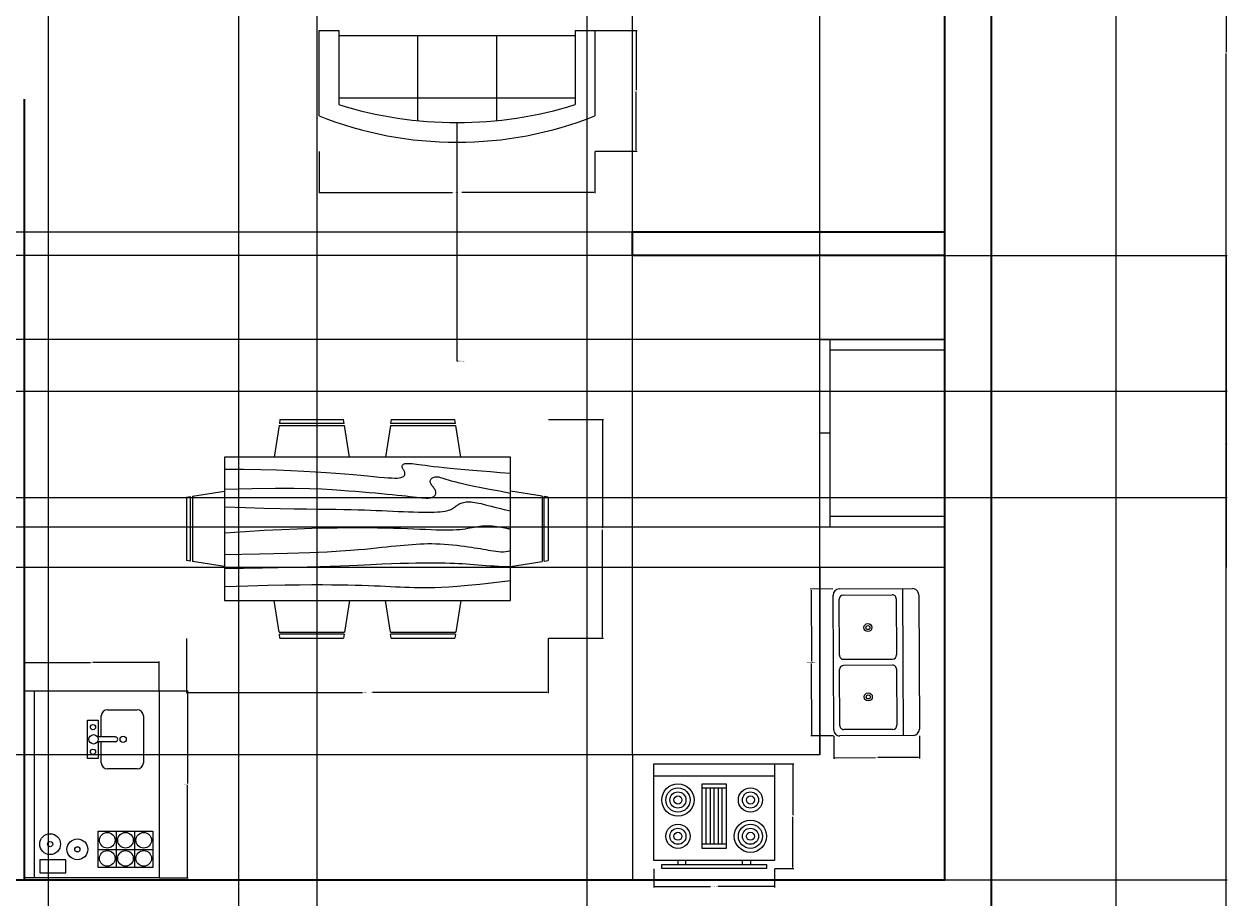
# Model space of a CAD drawing. Units: inches. Extents: x 109 to 572, y -157 to 568.
# Tile 4 of 5: x 341 to 572, y 192 to 360. Entities that reach past the tile are written whole.
import ezdxf

# ---------------------------------------------------------------- set-up
doc = ezdxf.new("R2010")
doc.units = ezdxf.units.IN
for name, color, linetype, lineweight in [('A-ANNO-DIMS', 2, 'Continuous', 18), ('A-EQPM', 9, 'Continuous', 18), ('A-FLOR-CASE', 32, 'Continuous', 18), ('A-FLOR-FIXT', 4, 'Continuous', 18), ('A-WALL', 7, 'Continuous', 35), ('C-PROP', 8, 'Continuous', 18), ('FURNUTURE', 50, 'Continuous', 18)]:
    doc.layers.add(name, color=color, linetype=linetype, lineweight=lineweight)
doc.styles.get("Standard").update_dxf_attribs({"font": 'arial.ttf'})
doc.dimstyles.get("Standard").update_dxf_attribs({"dimtxt": 0.18, "dimasz": 0.18, "dimexe": 0.18, "dimexo": 0.0625, "dimgap": 0.09, "dimtad": 0, "dimtih": 1, "dimtoh": 1, "dimdec": 4, "dimzin": 0, "dimdsep": 46, "dimtxsty": 'Standard', "dimcen": 0.09, "dimadec": 0, "dimazin": 0, "dimtfac": 1, "dimtdec": 4, "dimtofl": 0, "dimtmove": 0, "dimatfit": 3, "dimfxl": 1, "dimtolj": 1, "dimtzin": 0, "dimarcsym": 0})

# ---------------------------------------------------------------- blocks, each defined once
blk = doc.blocks.new('Sink-double - 36 in top')
for p, q in [((-18, -4), (18, -4)), ((-0.75, -18.5), (-0.75, -6.5)), ((0.75, -6.5), (0.75, -18.5))]:
    blk.add_line(p, q)
for points in [[(-16.5, 0), (16.5, 0)], [(-18, -19.5), (-18, -1.5)], [(18, -1.5), (18, -19.5)], [(-15.5, -5.5), (-1.75, -5.5)], [(1.75, -5.5), (15.5, -5.5)], [(-16.5, -18.5), (-16.5, -6.5)], [(16.5, -6.5), (16.5, -18.5)], [(-1.75, -19.5), (-15.5, -19.5)], [(15.5, -19.5), (1.75, -19.5)], [(16.5, -21), (-16.5, -21)]]:
    blk.add_lwpolyline(points)
for centre, radius in [((-8.5, -12.5), 1), ((8.5, -12.5), 1), ((-8.5, -12.5), 0.5), ((8.5, -12.5), 0.5)]:
    blk.add_circle(centre, radius)
for centre, radius, start, end in [((-16.5, -1.5), 1.5, 90, 180), ((16.5, -1.5), 1.5, 0, 90), ((-15.5, -6.5), 1, 90, 180), ((-1.75, -6.5), 1, 0, 90), ((1.75, -6.5), 1, 90, 180), ((15.5, -6.5), 1, 0, 90), ((-16.5, -19.5), 1.5, 180, 270), ((-15.5, -18.5), 1, 180, 270), ((-1.75, -18.5), 1, 270, 0), ((1.75, -18.5), 1, 180, 270), ((15.5, -18.5), 1, 270, 0), ((16.5, -19.5), 1.5, 270, 0)]:
    blk.add_arc(centre, radius, start, end)
blk = doc.blocks.new('Range-Oven - 30 in top')
for p, q in [((0, -3), (30, -3)), ((12, -6), (18, -6)), ((13, -20), (13, -6)), ((14, -6), (14, -20)), ((15, -20), (15, -6)), ((16, -6), (16, -20)), ((17, -20), (17, -6)), ((18, -20), (12, -20)), ((6, -24), (6, -25)), ((8, -25), (8, -24)), ((22, -25), (22, -24)), ((24, -24), (24, -25))]:
    blk.add_line(p, q)
for points in [[(0, -24), (0, 0), (30, 0), (30, -24)], [(12, -21), (12, -5), (18, -5), (18, -21)], [(2, -26), (2, -25), (28, -25), (28, -26)]]:
    blk.add_lwpolyline(points, close=True)
for centre, radius in [((6, -9), 4), ((6, -9), 3), ((6, -9), 2), ((6, -9), 1), ((24, -9), 3), ((24, -9), 2), ((24, -9), 1), ((24, -18), 4), ((6, -18), 3), ((6, -18), 2), ((6, -18), 1), ((24, -18), 3), ((24, -18), 2), ((24, -18), 1)]:
    blk.add_circle(centre, radius)
blk = doc.blocks.new('Sofa - Roundback 7 ft.')
for p, q in [((-12.00002, -32.4421), (-12.00003, -6.5971)), ((11.99997, -32.4421), (11.99998, -6.5971)), ((-36.000027, -34), (-36.000027, -11.4696)), ((-35.999844, -13.3819), (35.9998, -13.3819)), ((35.99998, -34), (35.99998, -11.4696)), ((-36.000027, -32.4421), (35.99998, -32.4421))]:
    blk.add_line(p, q)
for points in [[(-36.000027, -34), (-42.000027, -34), (-42.000027, -8)], [(41.99998, -8), (41.99998, -34), (35.99998, -34)]]:
    blk.add_lwpolyline(points)
for centre, radius, start, end in [((0, -114.25), 114.25, 68.43141, 111.5686), ((-0.00001, -127.1968), 121.1968, 72.72033, 107.2797)]:
    blk.add_arc(centre, radius, start, end)
blk = doc.blocks.new('Dining Set - 36 x 72 in.')
for p, q in [((-22, 27.5), (-22.1562, 26.50042)), ((-22, 27.5), (-6, 27.5)), ((-5.8437, 26.49966), (-6, 27.5)), ((6, 27.5), (5.8438, 26.50042)), ((6, 27.5), (22, 27.5)), ((22.1563, 26.49966), (22, 27.5)), ((-22.2343, 26.00059), (-23.4847, 17.99762)), ((-22.2304, 26), (-5.7608, 26)), ((-5.8416, 26.5), (-22.1534, 26.5)), ((-4.5152, 17.99762), (-5.7655, 25.99926)), ((5.7657, 26.00059), (4.5153, 17.99762)), ((5.7696, 26), (22.2392, 26)), ((22.1584, 26.5), (5.8466, 26.5)), ((23.4848, 17.99762), (22.2345, 25.99926)), ((36, 18), (-36, 18)), ((-36, 18), (-36, -18)), ((36, -18), (36, 18)), ((-44.0006, 8.23428), (-35.9976, 9.48474)), ((44.0006, 8.23428), (35.9976, 9.48474)), ((-45.5, 8), (-44.5004, 8.15617)), ((-45.5, 8), (-45.5, -8)), ((-44.5, -8.15843), (-44.5, 8.15338)), ((-44, 8.23041), (-44, -8.23915)), ((44, 8.23041), (44, -8.23915)), ((44.5, -8.15843), (44.5, 8.15338)), ((45.5, 8), (44.5005, 8.15617)), ((45.5, 8), (45.5, -8)), ((-44.4997, -8.15631), (-45.5, -8)), ((-35.9976, -9.48476), (-43.9993, -8.2345)), ((35.9976, -9.48476), (43.9993, -8.2345)), ((44.4997, -8.15631), (45.5, -8)), ((-36, -18), (36, -18)), ((-22.2343, -26.0006), (-23.4847, -17.99762)), ((-4.5152, -17.99762), (-5.7655, -25.99928)), ((5.7657, -26.0006), (4.5153, -17.99762)), ((23.4848, -17.99762), (22.2345, -25.99928)), ((-22.2304, -26), (-5.7608, -26)), ((-22, -27.5), (-22.1562, -26.50044)), ((-5.8416, -26.5), (-22.1534, -26.5)), ((-5.8437, -26.49967), (-6, -27.5)), ((5.7696, -26), (22.2392, -26)), ((6, -27.5), (5.8438, -26.50044)), ((22.1584, -26.5), (5.8466, -26.5)), ((22.1563, -26.49967), (22, -27.5)), ((-22, -27.5), (-6, -27.5)), ((6, -27.5), (22, -27.5))]:
    blk.add_line(p, q)
for points in [[(-36, 15), (-31.1772, 14.97754), (-26.8079, 14.91406), (-22.8538, 14.81543), (-19.276, 14.6875), (-16.0362, 14.53613), (-13.0957, 14.36718), (-10.4159, 14.18652), (-7.9583, 14), (-5.6904, 13.81315), (-3.6035, 13.63021), (-1.6954, 13.45508), (0.0365, 13.29166), (1.5945, 13.14388), (2.9811, 13.01562), (4.1988, 12.9108), (5.25, 12.83333), (6.1393, 12.78613), (6.8802, 12.76823), (7.4883, 12.77767), (7.9792, 12.8125), (8.3685, 12.87077), (8.6719, 12.95052), (8.9049, 13.0498), (9.0833, 13.16666), (9.2205, 13.29899), (9.3216, 13.44401), (9.3895, 13.59879), (9.4271, 13.76041), (9.4373, 13.92594), (9.4232, 14.09245), (9.3875, 14.257), (9.3333, 14.41666), (9.2638, 14.56917), (9.1836, 14.71484), (9.0975, 14.85465), (9.0104, 14.98958), (8.9272, 15.1206), (8.8529, 15.2487), (8.7922, 15.37483), (8.75, 15.5), (8.7305, 15.62467), (8.7344, 15.74739), (8.7617, 15.86621), (8.8125, 15.97916), (8.8867, 16.08431), (8.9844, 16.17968), (9.1055, 16.26334), (9.25, 16.33333), (9.4189, 16.38802), (9.6172, 16.42708), (9.8506, 16.45052), (10.125, 16.45833), (10.4463, 16.45052), (10.8203, 16.42708), (11.2529, 16.38802), (11.75, 16.33333), (12.3184, 16.26318), (12.9694, 16.17838), (13.7151, 16.07991), (14.5677, 15.96875), (15.5395, 15.84586), (16.6426, 15.71224), (17.8893, 15.56884), (19.2917, 15.41666), (20.859, 15.25667), (22.5879, 15.08984), (24.4721, 14.91715), (26.5052, 14.73958), (28.6809, 14.5581), (30.9929, 14.3737), (33.4347, 14.18733), (36, 14)], [(-36, 10), (-28.9766, 10.14274), (-23.1725, 10.20442), (-18.4241, 10.19775), (-14.5677, 10.13541), (-11.4399, 10.03011), (-8.877, 9.89453), (-6.7154, 9.74137), (-4.7917, 9.58333), (-2.9698, 9.43082), (-1.2246, 9.28515), (0.4415, 9.14534), (2.026, 9.01041), (3.5266, 8.87939), (4.9408, 8.7513), (6.266, 8.62516), (7.5, 8.5), (8.6411, 8.37549), (9.6914, 8.2539), (10.6538, 8.13818), (11.5312, 8.03125), (12.3267, 7.93603), (13.043, 7.85547), (13.6831, 7.79248), (14.25, 7.75), (14.7471, 7.7303), (15.1797, 7.73307), (15.5537, 7.75732), (15.875, 7.80208), (16.1494, 7.86637), (16.3828, 7.94922), (16.5811, 8.04964), (16.75, 8.16666), (16.8944, 8.29915), (17.0143, 8.44531), (17.1089, 8.60319), (17.1771, 8.77083), (17.218, 8.94629), (17.2305, 9.1276), (17.2137, 9.31282), (17.1667, 9.5), (17.0895, 9.6875), (16.987, 9.875), (16.8649, 10.0625), (16.7292, 10.25), (16.5856, 10.4375), (16.4401, 10.625), (16.2985, 10.8125), (16.1667, 11), (16.05, 11.18733), (15.9518, 11.3737), (15.8752, 11.5581), (15.8229, 11.73958), (15.798, 11.91715), (15.8034, 12.08984), (15.842, 12.25667), (15.9167, 12.41666), (16.0295, 12.56836), (16.1784, 12.70833), (16.3605, 12.83268), (16.5729, 12.9375), (16.8127, 13.01888), (17.0768, 13.07291), (17.3625, 13.0957), (17.6667, 13.08333), (17.9894, 13.03312), (18.3418, 12.94726), (18.7382, 12.82918), (19.1927, 12.68229), (19.7195, 12.51001), (20.3327, 12.31575), (21.0465, 12.10294), (21.875, 11.875), (22.8357, 11.63354), (23.959, 11.37304), (25.2786, 11.08618), (26.8282, 10.76562), (28.6414, 10.40405), (30.752, 9.99414), (33.1936, 9.52856), (36, 9)], [(-36, 5.5), (-30.7157, 5.3348), (-26.069, 5.20963), (-21.9946, 5.11767), (-18.4271, 5.05208), (-15.3009, 5.00602), (-12.5508, 4.97265), (-10.1112, 4.94515), (-7.9167, 4.91666), (-5.909, 4.88167), (-4.0586, 4.83984), (-2.3429, 4.79215), (-0.7396, 4.73958), (0.7739, 4.6831), (2.22, 4.6237), (3.6213, 4.56233), (5, 4.5), (6.373, 4.43782), (7.7344, 4.3776), (9.0723, 4.32129), (10.375, 4.27083), (11.6309, 4.22819), (12.8281, 4.19531), (13.9551, 4.17415), (15, 4.16666), (15.954, 4.17448), (16.819, 4.19791), (17.6001, 4.23698), (18.3021, 4.29166), (18.9299, 4.36198), (19.4883, 4.44791), (19.9823, 4.54948), (20.4167, 4.66666), (20.7969, 4.79899), (21.1302, 4.94401), (21.4245, 5.09879), (21.6875, 5.26041), (21.9271, 5.42594), (22.1511, 5.59245), (22.3672, 5.757), (22.5834, 5.91666), (22.8065, 6.06868), (23.0404, 6.21093), (23.2879, 6.34147), (23.5521, 6.45833), (23.8358, 6.55957), (24.142, 6.64323), (24.4735, 6.70735), (24.8334, 6.75), (25.2235, 6.76969), (25.642, 6.76692), (26.0858, 6.74267), (26.5521, 6.69791), (27.0379, 6.63362), (27.5404, 6.55078), (28.0565, 6.45036), (28.5834, 6.33333), (29.1242, 6.19987), (29.7071, 6.04687), (30.3661, 5.87044), (31.1354, 5.66666), (32.0493, 5.43164), (33.142, 5.16146), (34.4475, 4.85221), (36, 4.5)], [(-36, -1), (-30.7915, -0.6591), (-26.0195, -0.38216), (-21.6519, -0.16284), (-17.6563, 0.00521), (-14.0005, 0.12833), (-10.6523, 0.21289), (-7.5796, 0.26522), (-4.75, 0.29166), (-2.134, 0.29793), (0.2878, 0.28711), (2.5317, 0.26163), (4.6146, 0.22396), (6.5529, 0.17651), (8.3633, 0.12174), (10.0623, 0.06209), (11.6667, 0), (13.1899, -0.06201), (14.6341, -0.1211), (15.9982, -0.17432), (17.2813, -0.21875), (18.4823, -0.25147), (19.6003, -0.26953), (20.6343, -0.27002), (21.5834, -0.25), (22.4481, -0.20768), (23.2357, -0.14584), (23.9549, -0.06836), (24.6146, 0.02083), (25.2235, 0.11784), (25.7904, 0.21875), (26.3241, 0.31966), (26.8334, 0.41666), (27.3265, 0.50618), (27.8099, 0.58593), (28.2894, 0.65397), (28.7709, 0.70833), (29.2601, 0.74707), (29.763, 0.76823), (30.2855, 0.76985), (30.8334, 0.75), (31.4088, 0.70784), (31.9994, 0.64713), (32.589, 0.57275), (33.1615, 0.48958), (33.7008, 0.4025), (34.1908, 0.3164), (34.6153, 0.23616), (34.9584, 0.16666), (35.2099, 0.11165), (35.3848, 0.07031), (35.504, 0.04069), (35.5886, 0.02083), (35.6594, 0.00879), (35.7377, 0.0026), (35.8442, 0.00032), (36, 0)], [(-36, -6.5), (-27.1843, -6.31267), (-20.084, -6.1263), (-14.469, -5.9419), (-10.1094, -5.76042), (-6.7752, -5.58285), (-4.2363, -5.41016), (-2.2629, -5.24333), (-0.625, -5.08334), (0.8708, -4.93099), (2.2715, -4.78646), (3.5872, -4.64974), (4.8281, -4.52084), (6.0046, -4.39974), (7.127, -4.28646), (8.2053, -4.18099), (9.25, -4.08334), (10.2705, -3.99382), (11.2734, -3.91407), (12.2647, -3.84603), (13.25, -3.79167), (14.2354, -3.75293), (15.2266, -3.73177), (16.2295, -3.73015), (17.25, -3.75), (18.2912, -3.79248), (19.3451, -3.85547), (20.4009, -3.93604), (21.4479, -4.03125), (22.4754, -4.13819), (23.4727, -4.25391), (24.4289, -4.37549), (25.3334, -4.5), (26.1785, -4.62492), (26.9694, -4.74935), (27.7145, -4.87281), (28.4219, -4.99479), (29.1, -5.11483), (29.7572, -5.23242), (30.4016, -5.34709), (31.0417, -5.45834), (31.6837, -5.56437), (32.3262, -5.65821), (32.9658, -5.73153), (33.599, -5.77604), (34.2224, -5.78345), (34.8327, -5.74545), (35.4264, -5.65373), (36, -5.5)], [(-36, -10), (-26.4022, -9.81299), (-18.4675, -9.62891), (-11.9839, -9.45069), (-6.7396, -9.28125), (-2.5226, -9.12354), (0.8789, -8.98047), (3.6769, -8.85498), (6.0833, -8.75), (8.2767, -8.66765), (10.3021, -8.60677), (12.1712, -8.56543), (13.8958, -8.54167), (15.4876, -8.53353), (16.9583, -8.53907), (18.3197, -8.55632), (19.5834, -8.58334), (20.7616, -8.61841), (21.8685, -8.66081), (22.9188, -8.71004), (23.9271, -8.76563), (24.9081, -8.82707), (25.8763, -8.89388), (26.8465, -8.96558), (27.8334, -9.04167), (28.8474, -9.12118), (29.8828, -9.20117), (30.93, -9.27824), (31.9792, -9.34896), (33.0205, -9.40991), (34.0443, -9.45768), (35.0407, -9.48885), (36, -9.5)], [(-36, -14.5), (-30.0881, -14.33513), (-25.0332, -14.21224), (-20.7312, -14.12647), (-17.0781, -14.07292), (-13.97, -14.04671), (-11.3027, -14.04297), (-8.9724, -14.05681), (-6.875, -14.08334), (-4.9224, -14.11833), (-3.0905, -14.16016), (-1.3709, -14.20785), (0.2448, -14.26042), (1.7647, -14.3169), (3.1973, -14.3763), (4.5507, -14.43767), (5.8333, -14.5), (7.0554, -14.5621), (8.235, -14.62175), (9.3922, -14.67652), (10.5469, -14.72396), (11.7192, -14.76164), (12.929, -14.78711), (14.1965, -14.79794), (15.5417, -14.79167), (16.9933, -14.76424), (18.6152, -14.70508), (20.4804, -14.60197), (22.6615, -14.44271), (25.2312, -14.21509), (28.2624, -13.9069), (31.8277, -13.50594), (36, -13)]]:
    blk.add_lwpolyline(points)
blk = doc.blocks.new('Wet Bar')
for p, q in [((0, 0), (36, 0)), ((0, -26), (0, 0)), ((36, 0), (36, -26)), ((0, -2), (36, -2)), ((3.5, -3), (1, -3)), ((1, -3), (1, -8)), ((3.5, -8), (3.5, -3)), ((1, -8), (3.5, -8)), ((2, -14.25), (9, -14.25)), ((2, -24.75), (2, -14.25)), ((5.5, -14.25), (5.5, -24.75)), ((9, -14.25), (9, -24.75)), ((26.2, -17.55), (26.2, -14.1284)), ((27.1001, -17.55), (27.1001, -14.1284)), ((2, -17.75), (9, -17.75)), ((9, -21.25), (2, -21.25)), ((9, -24.75), (2, -24.75)), ((36, -26), (0, -26))]:
    blk.add_line(p, q)
for points in [[(26.2, -14.25), (22.95, -14.25), (22.95, -12.2), (26.75, -12.2)], [(26.7487, -12.2), (30.3501, -12.2), (30.3501, -14.25), (27.1001, -14.25)], [(20.95, -21.75), (20.95, -16.05)], [(22.15, -14.85), (26.2, -14.85)], [(27.1001, -14.85), (31.15, -14.85)], [(32.3501, -16.05), (32.3501, -21.75)], [(31.15, -22.95), (22.15, -22.95)]]:
    blk.add_lwpolyline(points)
for centre, radius in [((6.5, -5), 2), ((6.5, -5), 0.5), ((5.5, -10.25), 2), ((5.5, -10.25), 0.5), ((24.25, -13.25), 0.5), ((26.65, -13.35), 0.9), ((29, -13.25), 0.5), ((3.75, -16), 1.5), ((7.25, -16), 1.5), ((3.75, -19.5), 1.5), ((7.25, -19.5), 1.5), ((26.65, -19.05), 0.6), ((3.75, -23), 1.5), ((7.25, -23), 1.5)]:
    blk.add_circle(centre, radius)
for centre, radius, start, end in [((22.2251, -16.125), 1.2772, 93.36646, 176.6335), ((31.075, -16.125), 1.2772, 3.366461, 86.63354), ((26.65, -17.55), 0.45, 180, 0), ((22.2251, -21.675), 1.2772, 183.3665, 266.6335), ((31.075, -21.675), 1.2772, 273.3665, 356.6335)]:
    blk.add_arc(centre, radius, start, end)
blk = doc.blocks.new('*D19')
at = {"layer": 'A-ANNO-DIMS', "color": 0, "lineweight": -2, "transparency": 16777216}
for p, q in [((397.26, 335.57), (397.26, 327.5)), ((450.27, 335.57), (450.27, 327.5)), ((397.44, 327.68), (422.86, 327.68)), ((450.09, 327.68), (424.67, 327.68))]:
    blk.add_line(p, q, dxfattribs=at)
at = {"layer": 'A-ANNO-DIMS', "color": 0, "transparency": 16777216}
for points in [[(397.44, 327.71), (397.44, 327.65), (397.26, 327.68)], [(450.09, 327.71), (450.09, 327.65), (450.27, 327.68)]]:
    blk.add_solid(points, dxfattribs=at)
at = {"layer": 'Defpoints', "color": 0, "transparency": 16777216}
for p in [(397.26, 335.63), (450.27, 335.63), (397.26, 327.68)]:
    blk.add_point(p, dxfattribs=at)
at = {"layer": 'A-ANNO-DIMS', "color": 0, "transparency": 16777216, "insert": (423.76, 327.68), "char_height": 0.18, "attachment_point": 5}
blk.add_mtext('\\A1;SOFA 53 TYP.', dxfattribs=at)
blk = doc.blocks.new('*D20')
at = {"layer": 'A-ANNO-DIMS', "color": 0, "lineweight": -2, "transparency": 16777216}
for p, q in [((450.33, 358.78), (458.4, 358.78)), ((458.22, 358.6), (458.22, 347.39)), ((458.22, 335.81), (458.22, 347.02)), ((450.33, 335.63), (458.4, 335.63))]:
    blk.add_line(p, q, dxfattribs=at)
at = {"layer": 'A-ANNO-DIMS', "color": 0, "transparency": 16777216}
for points in [[(458.19, 358.6), (458.25, 358.6), (458.22, 358.78)], [(458.19, 335.81), (458.25, 335.81), (458.22, 335.63)]]:
    blk.add_solid(points, dxfattribs=at)
at = {"layer": 'Defpoints', "color": 0, "transparency": 16777216}
for p in [(450.27, 358.78), (450.27, 335.63), (458.22, 335.63)]:
    blk.add_point(p, dxfattribs=at)
at = {"layer": 'A-ANNO-DIMS', "color": 0, "transparency": 16777216, "insert": (458.22, 347.21), "char_height": 0.18, "attachment_point": 5}
blk.add_mtext('\\A1;23 TYP.', dxfattribs=at)
blk = doc.blocks.new('*D29')
at = {"layer": 'A-ANNO-DIMS', "color": 0, "lineweight": -2, "transparency": 16777216}
for p, q in [((495.99, 251.44), (491.64, 251.41)), ((491.82, 251.23), (491.89, 237.48)), ((491.96, 223.37), (491.89, 237.12)), ((496.14, 223.21), (491.78, 223.19))]:
    blk.add_line(p, q, dxfattribs=at)
at = {"layer": 'A-ANNO-DIMS', "color": 0, "transparency": 16777216}
for points in [[(491.85, 251.23), (491.79, 251.23), (491.82, 251.41)], [(491.99, 223.37), (491.93, 223.37), (491.96, 223.19)]]:
    blk.add_solid(points, dxfattribs=at)
at = {"layer": 'Defpoints', "color": 0, "transparency": 16777216}
for p in [(496.05, 251.44), (491.96, 223.19), (496.2, 223.21)]:
    blk.add_point(p, dxfattribs=at)
at = {"layer": 'A-ANNO-DIMS', "color": 0, "transparency": 16777216, "insert": (491.89, 237.3), "char_height": 0.18, "attachment_point": 5}
blk.add_mtext('\\A1;KITCHEN SINK 28', dxfattribs=at)
blk = doc.blocks.new('*D30')
at = {"layer": 'A-ANNO-DIMS', "color": 0, "lineweight": -2, "transparency": 16777216}
for p, q in [((496.2, 223.15), (496.22, 218.8)), ((512.66, 223.23), (512.69, 218.88)), ((496.4, 218.98), (504.24, 219.02)), ((512.5, 219.06), (504.66, 219.02))]:
    blk.add_line(p, q, dxfattribs=at)
at = {"layer": 'A-ANNO-DIMS', "color": 0, "transparency": 16777216}
for points in [[(496.4, 219.01), (496.4, 218.95), (496.22, 218.98)], [(512.5, 219.09), (512.51, 219.03), (512.68, 219.06)]]:
    blk.add_solid(points, dxfattribs=at)
at = {"layer": 'Defpoints', "color": 0, "transparency": 16777216}
for p in [(496.2, 223.21), (512.66, 223.3), (512.68, 219.06)]:
    blk.add_point(p, dxfattribs=at)
at = {"layer": 'A-ANNO-DIMS', "color": 0, "transparency": 16777216, "insert": (504.45, 219.02), "char_height": 0.18, "attachment_point": 5}
blk.add_mtext('\\A1;16', dxfattribs=at)
blk = doc.blocks.new('*D31')
at = {"layer": 'A-ANNO-DIMS', "color": 0, "lineweight": -2, "transparency": 16777216}
for p, q in [((461.58, 197.65), (461.58, 194.04)), ((484.82, 197.65), (484.82, 194.04)), ((461.76, 194.22), (472.51, 194.22)), ((484.64, 194.22), (473.9, 194.22))]:
    blk.add_line(p, q, dxfattribs=at)
at = {"layer": 'A-ANNO-DIMS', "color": 0, "transparency": 16777216}
for points in [[(461.76, 194.25), (461.76, 194.19), (461.58, 194.22)], [(484.64, 194.25), (484.64, 194.19), (484.82, 194.22)]]:
    blk.add_solid(points, dxfattribs=at)
at = {"layer": 'Defpoints', "color": 0, "transparency": 16777216}
for p in [(461.58, 197.71), (484.82, 197.71), (484.82, 194.22)]:
    blk.add_point(p, dxfattribs=at)
at = {"layer": 'A-ANNO-DIMS', "color": 0, "transparency": 16777216, "insert": (473.2, 194.22), "char_height": 0.18, "attachment_point": 5}
blk.add_mtext('\\A1;RANGE 23', dxfattribs=at)
blk = doc.blocks.new('*D32')
at = {"layer": 'A-ANNO-DIMS', "color": 0, "lineweight": -2, "transparency": 16777216}
for p, q in [((484.89, 217.85), (488.49, 217.85)), ((488.31, 217.67), (488.31, 207.96)), ((488.31, 197.89), (488.31, 207.6)), ((484.89, 197.71), (488.49, 197.71))]:
    blk.add_line(p, q, dxfattribs=at)
at = {"layer": 'A-ANNO-DIMS', "color": 0, "transparency": 16777216}
for points in [[(488.28, 217.67), (488.34, 217.67), (488.31, 217.85)], [(488.28, 197.89), (488.34, 197.89), (488.31, 197.71)]]:
    blk.add_solid(points, dxfattribs=at)
at = {"layer": 'Defpoints', "color": 0, "transparency": 16777216}
for p in [(484.82, 217.85), (488.31, 217.85), (484.82, 197.71)]:
    blk.add_point(p, dxfattribs=at)
at = {"layer": 'A-ANNO-DIMS', "color": 0, "transparency": 16777216, "insert": (488.31, 207.78), "char_height": 0.18, "attachment_point": 5}
blk.add_mtext('\\A1;20', dxfattribs=at)
blk = doc.blocks.new('*D33')
at = {"layer": 'A-ANNO-DIMS', "color": 0, "lineweight": -2, "transparency": 16777216}
for p, q in [((371.77, 241.93), (371.77, 231.39)), ((441.3, 241.93), (441.3, 231.39)), ((371.95, 231.57), (405.56, 231.57)), ((441.12, 231.57), (407.5, 231.57))]:
    blk.add_line(p, q, dxfattribs=at)
at = {"layer": 'A-ANNO-DIMS', "color": 0, "transparency": 16777216}
for points in [[(371.95, 231.6), (371.95, 231.54), (371.77, 231.57)], [(441.12, 231.6), (441.12, 231.54), (441.3, 231.57)]]:
    blk.add_solid(points, dxfattribs=at)
at = {"layer": 'Defpoints', "color": 0, "transparency": 16777216}
for p in [(371.77, 242), (441.3, 242), (441.3, 231.57)]:
    blk.add_point(p, dxfattribs=at)
at = {"layer": 'A-ANNO-DIMS', "color": 0, "transparency": 16777216, "insert": (406.53, 231.57), "char_height": 0.18, "attachment_point": 5}
blk.add_mtext('\\A1;DINING SET 70', dxfattribs=at)
blk = doc.blocks.new('*D34')
at = {"layer": 'A-ANNO-DIMS', "color": 0, "lineweight": -2, "transparency": 16777216}
for p, q in [((441.36, 284.02), (451.91, 284.02)), ((451.73, 283.84), (451.73, 263.19)), ((451.73, 242.18), (451.73, 262.83)), ((441.36, 242), (451.91, 242))]:
    blk.add_line(p, q, dxfattribs=at)
at = {"layer": 'A-ANNO-DIMS', "color": 0, "transparency": 16777216}
for points in [[(451.7, 283.84), (451.76, 283.84), (451.73, 284.02)], [(451.7, 242.18), (451.76, 242.18), (451.73, 242)]]:
    blk.add_solid(points, dxfattribs=at)
at = {"layer": 'Defpoints', "color": 0, "transparency": 16777216}
for p in [(441.3, 284.02), (451.73, 284.02), (441.3, 242)]:
    blk.add_point(p, dxfattribs=at)
at = {"layer": 'A-ANNO-DIMS', "color": 0, "transparency": 16777216, "insert": (451.73, 263.01), "char_height": 0.18, "attachment_point": 5}
blk.add_mtext('\\A1;42', dxfattribs=at)
blk = doc.blocks.new('*D35')
at = {"layer": 'A-ANNO-DIMS', "color": 0, "lineweight": -2, "transparency": 16777216}
for p, q in [((366.58, 231.89), (372.1, 231.89)), ((371.92, 231.71), (371.92, 214.07)), ((371.92, 196.07), (371.92, 213.71)), ((366.58, 195.89), (372.1, 195.89))]:
    blk.add_line(p, q, dxfattribs=at)
at = {"layer": 'A-ANNO-DIMS', "color": 0, "transparency": 16777216}
for points in [[(371.89, 231.71), (371.95, 231.71), (371.92, 231.89)], [(371.89, 196.07), (371.95, 196.07), (371.92, 195.89)]]:
    blk.add_solid(points, dxfattribs=at)
at = {"layer": 'Defpoints', "color": 0, "transparency": 16777216}
for p in [(366.52, 231.89), (371.92, 231.89), (366.52, 195.89)]:
    blk.add_point(p, dxfattribs=at)
at = {"layer": 'A-ANNO-DIMS', "color": 0, "transparency": 16777216, "insert": (371.92, 213.89), "char_height": 0.18, "attachment_point": 5}
blk.add_mtext('\\A1;WET BAR 36', dxfattribs=at)
blk = doc.blocks.new('*D36')
at = {"layer": 'A-ANNO-DIMS', "color": 0, "lineweight": -2, "transparency": 16777216}
for p, q in [((340.52, 231.95), (340.52, 237.47)), ((340.7, 237.29), (353.3, 237.29)), ((366.34, 237.29), (353.74, 237.29)), ((366.52, 231.95), (366.52, 237.47))]:
    blk.add_line(p, q, dxfattribs=at)
at = {"layer": 'A-ANNO-DIMS', "color": 0, "transparency": 16777216}
for points in [[(340.7, 237.32), (340.7, 237.26), (340.52, 237.29)], [(366.34, 237.32), (366.34, 237.26), (366.52, 237.29)]]:
    blk.add_solid(points, dxfattribs=at)
at = {"layer": 'Defpoints', "color": 0, "transparency": 16777216}
for p in [(340.52, 237.29), (340.52, 231.89), (366.52, 231.89)]:
    blk.add_point(p, dxfattribs=at)
at = {"layer": 'A-ANNO-DIMS', "color": 0, "transparency": 16777216, "insert": (353.52, 237.29), "char_height": 0.18, "attachment_point": 5}
blk.add_mtext('\\A1;26', dxfattribs=at)
blk = doc.blocks.new('*D44')
at = {"layer": 'A-ANNO-DIMS', "color": 0, "lineweight": -2, "transparency": 16777216}
for p, q in [((526.58, 522.54), (571.85, 522.54)), ((571.67, 522.36), (571.67, 354.72)), ((571.67, 186.72), (571.67, 354.36)), ((526.58, 186.54), (571.85, 186.54))]:
    blk.add_line(p, q, dxfattribs=at)
at = {"layer": 'A-ANNO-DIMS', "color": 0, "transparency": 16777216}
for points in [[(571.64, 522.36), (571.7, 522.36), (571.67, 522.54)], [(571.64, 186.72), (571.7, 186.72), (571.67, 186.54)]]:
    blk.add_solid(points, dxfattribs=at)
at = {"layer": 'Defpoints', "color": 0, "transparency": 16777216}
for p in [(526.52, 522.54), (571.67, 522.54), (526.52, 186.54)]:
    blk.add_point(p, dxfattribs=at)
at = {"layer": 'A-ANNO-DIMS', "color": 0, "transparency": 16777216, "insert": (571.67, 354.54), "char_height": 0.18, "attachment_point": 5}
blk.add_mtext('\\A1;336', dxfattribs=at)
blk = doc.blocks.new('*D52')
at = {"layer": 'A-ANNO-DIMS', "color": 0, "lineweight": -2, "transparency": 16777216}
for p, q in [((517.58, 315.54), (571.85, 315.54)), ((571.67, 315.36), (571.67, 255.72)), ((571.67, 195.72), (571.67, 255.36)), ((517.58, 195.54), (571.85, 195.54))]:
    blk.add_line(p, q, dxfattribs=at)
at = {"layer": 'A-ANNO-DIMS', "color": 0, "transparency": 16777216}
for points in [[(571.64, 315.36), (571.7, 315.36), (571.67, 315.54)], [(571.64, 195.72), (571.7, 195.72), (571.67, 195.54)]]:
    blk.add_solid(points, dxfattribs=at)
at = {"layer": 'Defpoints', "color": 0, "transparency": 16777216}
for p in [(517.52, 315.54), (571.67, 315.54), (517.52, 195.54)]:
    blk.add_point(p, dxfattribs=at)
at = {"layer": 'A-ANNO-DIMS', "color": 0, "transparency": 16777216, "insert": (571.67, 255.54), "char_height": 0.18, "attachment_point": 5}
blk.add_mtext('\\A1;120', dxfattribs=at)
blk = doc.blocks.new('*D53')
at = {"layer": 'A-ANNO-DIMS', "color": 0, "lineweight": -2, "transparency": 16777216}
for p, q in [((457.52, 320.1), (457.52, 567.87)), ((457.7, 567.69), (487.3, 567.69)), ((517.34, 567.69), (487.74, 567.69)), ((517.52, 320.1), (517.52, 567.87))]:
    blk.add_line(p, q, dxfattribs=at)
at = {"layer": 'A-ANNO-DIMS', "color": 0, "transparency": 16777216}
for points in [[(457.7, 567.72), (457.7, 567.66), (457.52, 567.69)], [(517.34, 567.72), (517.34, 567.66), (517.52, 567.69)]]:
    blk.add_solid(points, dxfattribs=at)
at = {"layer": 'Defpoints', "color": 0, "transparency": 16777216}
for p in [(517.52, 567.69), (457.52, 320.04), (517.52, 320.04)]:
    blk.add_point(p, dxfattribs=at)
at = {"layer": 'A-ANNO-DIMS', "color": 0, "transparency": 16777216, "insert": (487.52, 567.69), "char_height": 0.18, "attachment_point": 5}
blk.add_mtext('\\A1;60', dxfattribs=at)
blk = doc.blocks.new('*D54')
at = {"layer": 'A-ANNO-DIMS', "color": 0, "lineweight": -2, "transparency": 16777216}
for p, q in [((493.52, 299.47), (493.52, 567.87)), ((493.7, 567.69), (505.3, 567.69)), ((517.34, 567.69), (505.74, 567.69)), ((517.52, 299.47), (517.52, 567.87))]:
    blk.add_line(p, q, dxfattribs=at)
at = {"layer": 'A-ANNO-DIMS', "color": 0, "transparency": 16777216}
for points in [[(493.7, 567.72), (493.7, 567.66), (493.52, 567.69)], [(517.34, 567.72), (517.34, 567.66), (517.52, 567.69)]]:
    blk.add_solid(points, dxfattribs=at)
at = {"layer": 'Defpoints', "color": 0, "transparency": 16777216}
for p in [(517.52, 567.69), (493.52, 299.4), (517.52, 299.4)]:
    blk.add_point(p, dxfattribs=at)
at = {"layer": 'A-ANNO-DIMS', "color": 0, "transparency": 16777216, "insert": (505.52, 567.69), "char_height": 0.18, "attachment_point": 5}
blk.add_mtext('\\A1;24', dxfattribs=at)
blk = doc.blocks.new('*D55')
at = {"layer": 'A-ANNO-DIMS', "color": 0, "lineweight": -2, "transparency": 16777216}
for p, q in [((493.46, 299.4), (109.19, 299.4)), ((109.37, 299.22), (109.37, 281.56)), ((109.37, 263.53), (109.37, 281.2)), ((493.46, 263.35), (109.19, 263.35))]:
    blk.add_line(p, q, dxfattribs=at)
at = {"layer": 'A-ANNO-DIMS', "color": 0, "transparency": 16777216}
for points in [[(109.34, 299.22), (109.4, 299.22), (109.37, 299.4)], [(109.34, 263.53), (109.4, 263.53), (109.37, 263.35)]]:
    blk.add_solid(points, dxfattribs=at)
at = {"layer": 'Defpoints', "color": 0, "transparency": 16777216}
for p in [(109.37, 299.4), (493.52, 299.4), (493.52, 263.35)]:
    blk.add_point(p, dxfattribs=at)
at = {"layer": 'A-ANNO-DIMS', "color": 0, "transparency": 16777216, "insert": (109.37, 281.38), "char_height": 0.18, "attachment_point": 5}
blk.add_mtext('\\A1;36.05', dxfattribs=at)
blk = doc.blocks.new('*D56')
at = {"layer": 'A-ANNO-DIMS', "color": 0, "lineweight": -2, "transparency": 16777216}
for p, q in [((493.46, 255.54), (109.19, 255.54)), ((109.37, 255.36), (109.37, 237.72)), ((109.37, 219.72), (109.37, 237.36)), ((493.46, 219.54), (109.19, 219.54))]:
    blk.add_line(p, q, dxfattribs=at)
at = {"layer": 'A-ANNO-DIMS', "color": 0, "transparency": 16777216}
for points in [[(109.34, 255.36), (109.4, 255.36), (109.37, 255.54)], [(109.34, 219.72), (109.4, 219.72), (109.37, 219.54)]]:
    blk.add_solid(points, dxfattribs=at)
at = {"layer": 'Defpoints', "color": 0, "transparency": 16777216}
for p in [(493.52, 255.54), (109.37, 219.54), (493.52, 219.54)]:
    blk.add_point(p, dxfattribs=at)
at = {"layer": 'A-ANNO-DIMS', "color": 0, "transparency": 16777216, "insert": (109.37, 237.54), "char_height": 0.18, "attachment_point": 5}
blk.add_mtext('\\A1;36', dxfattribs=at)
blk = doc.blocks.new('*D61')
at = {"layer": 'A-ANNO-DIMS', "color": 0, "lineweight": -2, "transparency": 16777216}
for p, q in [((396.8, 428.71), (396.8, 105.21)), ((448.7, 428.71), (448.7, 105.21)), ((396.98, 105.39), (422.43, 105.39)), ((448.52, 105.39), (423.08, 105.39))]:
    blk.add_line(p, q, dxfattribs=at)
at = {"layer": 'A-ANNO-DIMS', "color": 0, "transparency": 16777216}
for points in [[(396.98, 105.42), (396.98, 105.36), (396.8, 105.39)], [(448.52, 105.42), (448.52, 105.36), (448.7, 105.39)]]:
    blk.add_solid(points, dxfattribs=at)
at = {"layer": 'Defpoints', "color": 0, "transparency": 16777216}
for p in [(396.8, 428.77), (448.7, 428.77), (448.7, 105.39)]:
    blk.add_point(p, dxfattribs=at)
at = {"layer": 'A-ANNO-DIMS', "color": 0, "transparency": 16777216, "insert": (422.75, 105.39), "char_height": 0.18, "attachment_point": 5}
blk.add_mtext('\\A1;51.9', dxfattribs=at)
blk = doc.blocks.new('*D63')
at = {"layer": 'A-ANNO-DIMS', "color": 0, "lineweight": -2, "transparency": 16777216}
for p, q in [((457.46, 320.04), (109.19, 320.04)), ((109.37, 319.86), (109.37, 317.97)), ((109.37, 315.72), (109.37, 317.61)), ((457.46, 315.54), (109.19, 315.54))]:
    blk.add_line(p, q, dxfattribs=at)
at = {"layer": 'A-ANNO-DIMS', "color": 0, "transparency": 16777216}
for points in [[(109.34, 319.86), (109.4, 319.86), (109.37, 320.04)], [(109.34, 315.72), (109.4, 315.72), (109.37, 315.54)]]:
    blk.add_solid(points, dxfattribs=at)
at = {"layer": 'Defpoints', "color": 0, "transparency": 16777216}
for p in [(109.37, 320.04), (457.52, 320.04), (457.52, 315.54)]:
    blk.add_point(p, dxfattribs=at)
at = {"layer": 'A-ANNO-DIMS', "color": 0, "transparency": 16777216, "insert": (109.37, 317.79), "char_height": 0.18, "attachment_point": 5}
blk.add_mtext('\\A1;4.5', dxfattribs=at)
blk = doc.blocks.new('*D66')
at = {"layer": 'A-ANNO-DIMS', "color": 0, "lineweight": -2, "transparency": 16777216}
for p, q in [((457.52, 219.6), (457.52, 567.87)), ((457.7, 567.69), (475.3, 567.69)), ((493.34, 567.69), (475.74, 567.69)), ((493.52, 219.6), (493.52, 567.87))]:
    blk.add_line(p, q, dxfattribs=at)
at = {"layer": 'A-ANNO-DIMS', "color": 0, "transparency": 16777216}
for points in [[(457.7, 567.72), (457.7, 567.66), (457.52, 567.69)], [(493.34, 567.72), (493.34, 567.66), (493.52, 567.69)]]:
    blk.add_solid(points, dxfattribs=at)
at = {"layer": 'Defpoints', "color": 0, "transparency": 16777216}
for p in [(493.52, 567.69), (457.52, 219.54), (493.52, 219.54)]:
    blk.add_point(p, dxfattribs=at)
at = {"layer": 'A-ANNO-DIMS', "color": 0, "transparency": 16777216, "insert": (475.52, 567.69), "char_height": 0.18, "attachment_point": 5}
blk.add_mtext('\\A1;36', dxfattribs=at)
blk = doc.blocks.new('*D67')
at = {"layer": 'A-ANNO-DIMS', "color": 0, "lineweight": -2, "transparency": 16777216}
for p, q in [((457.46, 219.54), (109.19, 219.54)), ((109.37, 219.36), (109.37, 207.72)), ((109.37, 195.72), (109.37, 207.36)), ((457.46, 195.54), (109.19, 195.54))]:
    blk.add_line(p, q, dxfattribs=at)
at = {"layer": 'A-ANNO-DIMS', "color": 0, "transparency": 16777216}
for points in [[(109.34, 219.36), (109.4, 219.36), (109.37, 219.54)], [(109.34, 195.72), (109.4, 195.72), (109.37, 195.54)]]:
    blk.add_solid(points, dxfattribs=at)
at = {"layer": 'Defpoints', "color": 0, "transparency": 16777216}
for p in [(457.52, 219.54), (109.37, 195.54), (457.52, 195.54)]:
    blk.add_point(p, dxfattribs=at)
at = {"layer": 'A-ANNO-DIMS', "color": 0, "transparency": 16777216, "insert": (109.37, 207.54), "char_height": 0.18, "attachment_point": 5}
blk.add_mtext('\\A1;24', dxfattribs=at)
blk = doc.blocks.new('*D69')
at = {"layer": 'A-ANNO-DIMS', "color": 0, "lineweight": -2, "transparency": 16777216}
for p, q in [((216.08, 289.49), (571.85, 289.49)), ((571.67, 289.31), (571.67, 279.45)), ((571.67, 269.22), (571.67, 279.08)), ((216.08, 269.04), (571.85, 269.04))]:
    blk.add_line(p, q, dxfattribs=at)
at = {"layer": 'A-ANNO-DIMS', "color": 0, "transparency": 16777216}
for points in [[(571.64, 289.31), (571.7, 289.31), (571.67, 289.49)], [(571.64, 269.22), (571.7, 269.22), (571.67, 269.04)]]:
    blk.add_solid(points, dxfattribs=at)
at = {"layer": 'Defpoints', "color": 0, "transparency": 16777216}
for p in [(216.02, 289.49), (571.67, 289.49), (216.02, 269.04)]:
    blk.add_point(p, dxfattribs=at)
at = {"layer": 'A-ANNO-DIMS', "color": 0, "transparency": 16777216, "insert": (571.67, 279.26), "char_height": 0.18, "attachment_point": 5}
blk.add_mtext('\\A1;20.45', dxfattribs=at)
blk = doc.blocks.new('*D70')
at = {"layer": 'A-ANNO-DIMS', "color": 0, "lineweight": -2, "transparency": 16777216}
for p, q in [((517.46, 315.54), (109.19, 315.54)), ((109.37, 315.36), (109.37, 307.65)), ((109.37, 299.58), (109.37, 307.29)), ((517.46, 299.4), (109.19, 299.4))]:
    blk.add_line(p, q, dxfattribs=at)
at = {"layer": 'A-ANNO-DIMS', "color": 0, "transparency": 16777216}
for points in [[(109.34, 315.36), (109.4, 315.36), (109.37, 315.54)], [(109.34, 299.58), (109.4, 299.58), (109.37, 299.4)]]:
    blk.add_solid(points, dxfattribs=at)
at = {"layer": 'Defpoints', "color": 0, "transparency": 16777216}
for p in [(517.52, 315.54), (109.37, 299.4), (517.52, 299.4)]:
    blk.add_point(p, dxfattribs=at)
at = {"layer": 'A-ANNO-DIMS', "color": 0, "transparency": 16777216, "insert": (109.37, 307.47), "char_height": 0.18, "attachment_point": 5}
blk.add_mtext('\\A1;16.136', dxfattribs=at)
blk = doc.blocks.new('*D71')
at = {"layer": 'A-ANNO-DIMS', "color": 0, "lineweight": -2, "transparency": 16777216}
for p, q in [((345.17, 436.98), (345.17, 105.21)), ((381.74, 436.98), (381.74, 105.21)), ((345.35, 105.39), (363.06, 105.39)), ((381.56, 105.39), (363.85, 105.39))]:
    blk.add_line(p, q, dxfattribs=at)
at = {"layer": 'A-ANNO-DIMS', "color": 0, "transparency": 16777216}
for points in [[(345.35, 105.42), (345.35, 105.36), (345.17, 105.39)], [(381.56, 105.42), (381.56, 105.36), (381.74, 105.39)]]:
    blk.add_solid(points, dxfattribs=at)
at = {"layer": 'Defpoints', "color": 0, "transparency": 16777216}
for p in [(345.17, 437.04), (381.74, 437.04), (381.74, 105.39)]:
    blk.add_point(p, dxfattribs=at)
at = {"layer": 'A-ANNO-DIMS', "color": 0, "transparency": 16777216, "insert": (363.46, 105.39), "char_height": 0.18, "attachment_point": 5}
blk.add_mtext('\\A1;36.57', dxfattribs=at)
blk = doc.blocks.new('*D73')
at = {"layer": 'A-ANNO-DIMS', "color": 0, "lineweight": -2, "transparency": 16777216}
for p, q in [((423.67, 417.59), (423.85, 417.59)), ((423.76, 417.5), (423.76, 417.68)), ((423.77, 295.21), (423.77, 340.92)), ((423.95, 295.21), (423.77, 295.21))]:
    blk.add_line(p, q, dxfattribs=at)
at = {"layer": 'A-ANNO-DIMS', "color": 0, "transparency": 16777216}
blk.add_solid([(423.8, 340.92), (423.74, 340.92), (423.77, 341.1)], dxfattribs=at)
at = {"layer": 'Defpoints', "color": 0, "transparency": 16777216}
for p in [(423.76, 417.59), (423.77, 341.1)]:
    blk.add_point(p, dxfattribs=at)
at = {"layer": 'A-ANNO-DIMS', "color": 0, "transparency": 16777216, "insert": (424.62, 295.21), "char_height": 0.18, "attachment_point": 5}
blk.add_mtext('\\A1;2X R76.49', dxfattribs=at)

msp = doc.modelspace()

# ---------------------------------------------------------------- linework, layer by layer
at = {"layer": 'A-EQPM'}
for p, q in [((493.5195, 263.3515), (493.5195, 299.4036)), ((493.5195, 299.4036), (517.5195, 299.4036)), ((495.5195, 263.3515), (495.5195, 299.4036)), ((495.5195, 297.4036), (517.5195, 297.4036)), ((495.5195, 281.3775), (493.5195, 281.3775)), ((517.5195, 265.3515), (495.5195, 265.3515)), ((517.5195, 263.3515), (493.5195, 263.3515))]:
    msp.add_line(p, q, dxfattribs=at)
at = {"layer": 'A-FLOR-CASE'}
for p, q in [((517.5195, 255.5398), (493.5195, 255.5398)), ((493.5195, 255.5398), (493.5195, 219.5398)), ((493.5195, 219.5398), (457.5195, 219.5398)), ((457.5195, 219.5398), (457.5195, 195.5398))]:
    msp.add_line(p, q, dxfattribs=at)
at = {"layer": 'A-WALL'}
for p, q in [((526.5195, 186.5398), (526.5195, 522.5398)), ((517.5195, 195.5398), (517.5195, 513.5398)), ((340.5195, 345.6055), (340.5195, 195.5398)), ((517.5195, 320.0398), (457.5195, 320.0398)), ((457.5195, 315.5398), (457.5195, 320.0398)), ((517.5195, 315.5398), (457.5195, 315.5398)), ((211.5195, 195.5398), (517.5195, 195.5398))]:
    msp.add_line(p, q, dxfattribs=at)
at = {"layer": 'C-PROP'}
msp.add_line((550.5195, 126.5398), (550.5195, 546.5398), dxfattribs=at)

# ---------------------------------------------------------------- block references
at = {"layer": 'A-EQPM', "xscale": 0.7747134510318094, "yscale": 0.7747134510318094, "zscale": 0.7747134510318094}
msp.add_blockref('Range-Oven - 30 in top', (461.5811, 217.8502), dxfattribs=at)
at = {"layer": 'A-FLOR-CASE', "rotation": 90}
msp.add_blockref('Wet Bar', (340.5195, 195.8885), dxfattribs=at)
at = {"layer": 'A-FLOR-FIXT', "xscale": 0.7840589504409365, "yscale": 0.7840589504409365, "zscale": 0.7840589504409365, "rotation": 270.2996233216522}
msp.add_blockref('Sink-double - 36 in top', (512.589, 237.4088), dxfattribs=at)
at = {"layer": 'FURNUTURE', "xscale": 0.6311149755578328, "yscale": 0.6311149755578328, "zscale": 0.6311149755578328, "rotation": 180}
msp.add_blockref('Sofa - Roundback 7 ft.', (423.7646, 337.3176), dxfattribs=at)
at = {"layer": 'FURNUTURE', "xscale": 0.7640934223430186, "yscale": 0.7640934223430186, "zscale": 0.7640934223430186}
msp.add_blockref('Dining Set - 36 x 72 in.', (406.5335, 263.0094), dxfattribs=at)

# ---------------------------------------------------------------- dimensions: what is measured, and where the dimension line sits
at = {"layer": 'A-ANNO-DIMS'}
for base, p1, p2, override, picture, middle in [((517.5195, 567.6898), (457.5195, 320.0398), (517.5195, 320.0398), {"dimdec": 0, "dimlfac": 1, "dimrnd": 0, "dimzin": 0, "dimdsep": 46, "dimlunit": 2}, '*D53', (487.5195, 567.6898)), ((493.5195, 567.6898), (457.5195, 219.5398), (493.5195, 219.5398), {"dimdec": 0, "dimlfac": 1, "dimrnd": 0, "dimzin": 0, "dimdsep": 46, "dimlunit": 2}, '*D66', (475.5195, 567.6898)), ((517.5195, 567.6898), (493.5195, 299.4036), (517.5195, 299.4036), {"dimdec": 0, "dimlfac": 1, "dimrnd": 0, "dimzin": 0, "dimdsep": 46, "dimlunit": 2}, '*D54', (505.5195, 567.6898)), ((381.7416, 105.3898), (345.1719, 437.0398), (381.7416, 437.0398), {"dimdec": 2, "dimlfac": 1, "dimrnd": 0, "dimzin": 0, "dimdsep": 46, "dimlunit": 2}, '*D71', (363.4567, 105.3898)), ((448.7025, 105.3898), (396.8044, 428.7734), (448.7025, 428.7734), {"dimdec": 1, "dimlfac": 1, "dimrnd": 0, "dimzin": 0, "dimdsep": 46, "dimlunit": 2}, '*D61', (422.7534, 105.3898))]:
    dim = msp.add_linear_dim(base=base, p1=p1, p2=p2, dimstyle='Standard', override=override, dxfattribs=at)
    dim.commit()
    dim.dimension.update_dxf_attribs({"geometry": picture, "text_midpoint": middle})
for base, p1, p2, angle, override, picture, middle in [((571.6695, 522.5398), (526.5195, 186.5398), (526.5195, 522.5398), 90, {"dimdec": 0, "dimlfac": 1, "dimrnd": 0, "dimzin": 0, "dimdsep": 46, "dimlunit": 2}, '*D44', (571.6695, 354.5398)), ((109.3695, 320.0398), (457.5195, 315.5398), (457.5195, 320.0398), 90, {"dimdec": 1, "dimlfac": 1, "dimrnd": 0, "dimzin": 0, "dimdsep": 46, "dimlunit": 2}, '*D63', (109.3695, 317.7898)), ((109.3695, 299.4036), (517.5195, 315.5398), (517.5195, 299.4036), 90, {"dimdec": 3, "dimlfac": 1, "dimrnd": 0, "dimzin": 0, "dimdsep": 46, "dimlunit": 2}, '*D70', (109.3695, 307.4717)), ((571.6695, 315.5398), (517.5195, 195.5398), (517.5195, 315.5398), 90, {"dimdec": 0, "dimlfac": 1, "dimrnd": 0, "dimzin": 0, "dimdsep": 46, "dimlunit": 2}, '*D52', (571.6695, 255.5398)), ((109.3695, 299.4036), (493.5195, 263.3515), (493.5195, 299.4036), 90, {"dimdec": 2, "dimlfac": 1, "dimrnd": 0, "dimzin": 0, "dimdsep": 46, "dimlunit": 2}, '*D55', (109.3695, 281.3775)), ((571.6695, 289.4894), (216.0195, 269.0398), (216.0195, 289.4894), 90, {"dimdec": 2, "dimlfac": 1, "dimrnd": 0, "dimzin": 0, "dimdsep": 46, "dimlunit": 2}, '*D69', (571.6695, 279.2646)), ((451.7296, 284.0219), (441.2997, 241.9968), (441.2997, 284.0219), 90, {"dimdec": 0, "dimlfac": 1, "dimrnd": 0, "dimzin": 0, "dimdsep": 46, "dimlunit": 2}, '*D34', (451.7296, 263.0094)), ((109.3695, 219.5398), (493.5195, 255.5398), (493.5195, 219.5398), 90, {"dimdec": 0, "dimlfac": 1, "dimrnd": 0, "dimzin": 0, "dimdsep": 46, "dimlunit": 2}, '*D56', (109.3695, 237.5398)), ((340.5195, 237.2885), (366.5195, 231.8885), (340.5195, 231.8885), 180, {"dimdec": 0, "dimlfac": 1, "dimrnd": 0, "dimzin": 0, "dimdsep": 46, "dimlunit": 2}, '*D36', (353.5195, 237.2885)), ((512.685, 219.0621), (496.1978, 223.2098), (512.6629, 223.296), 0.299623, {"dimdec": 0, "dimlfac": 1, "dimrnd": 0, "dimzin": 0, "dimdsep": 46, "dimlunit": 2}, '*D30', (504.4525, 219.019)), ((109.3695, 195.5398), (457.5195, 219.5398), (457.5195, 195.5398), 90, {"dimdec": 0, "dimlfac": 1, "dimrnd": 0, "dimzin": 0, "dimdsep": 46, "dimlunit": 2}, '*D67', (109.3695, 207.5398)), ((488.3087, 217.8502), (484.8225, 197.7077), (484.8225, 217.8502), 90, {"dimdec": 0, "dimlfac": 1, "dimrnd": 0, "dimzin": 0, "dimdsep": 46, "dimlunit": 2}, '*D32', (488.3087, 207.7789))]:
    dim = msp.add_linear_dim(base=base, p1=p1, p2=p2, angle=angle, dimstyle='Standard', override=override, dxfattribs=at)
    dim.commit()
    dim.dimension.update_dxf_attribs({"geometry": picture, "text_midpoint": middle})
dim = msp.add_radius_dim(center=(423.7646, 417.5934), mpoint=(423.765, 341.1043), text='2X <>', dimstyle='Standard', override={"dimdec": 2, "dimlfac": 1, "dimrnd": 0, "dimzin": 0, "dimdsep": 46, "dimlunit": 2}, dxfattribs=at)
dim.commit()
dim.dimension.update_dxf_attribs({"geometry": '*D73', "text_midpoint": (424.6202, 295.2108), "dimtype": 164})
for base, p1, p2, angle, text, picture, middle in [((458.2235, 335.6346), (450.2715, 358.7755), (450.2715, 335.6346), 270, '<> TYP.', '*D20', (458.2235, 347.2051)), ((397.2578, 327.6826), (450.2715, 335.6346), (397.2578, 335.6346), 180, 'SOFA <> TYP.', '*D19', (423.7646, 327.6826)), ((491.964, 223.1877), (496.0502, 251.4356), (496.1978, 223.2098), 270.299623, 'KITCHEN SINK <>', '*D29', (491.8902, 237.3006)), ((371.9195, 231.8885), (366.5195, 195.8885), (366.5195, 231.8885), 90, 'WET BAR <>', '*D35', (371.9195, 213.8885))]:
    dim = msp.add_linear_dim(base=base, p1=p1, p2=p2, angle=angle, text=text, dimstyle='Standard', override={"dimdec": 0, "dimlfac": 1, "dimrnd": 0, "dimzin": 0, "dimdsep": 46, "dimlunit": 2}, dxfattribs=at)
    dim.commit()
    dim.dimension.update_dxf_attribs({"geometry": picture, "text_midpoint": middle})
for base, p1, p2, text, picture, middle in [((441.2997, 231.5669), (371.7672, 241.9968), (441.2997, 241.9968), 'DINING SET <>', '*D33', (406.5335, 231.5669)), ((484.8225, 194.2214), (461.5811, 197.7077), (484.8225, 197.7077), 'RANGE <>', '*D31', (473.2018, 194.2214))]:
    dim = msp.add_linear_dim(base=base, p1=p1, p2=p2, text=text, dimstyle='Standard', override={"dimdec": 0, "dimlfac": 1, "dimrnd": 0, "dimzin": 0, "dimdsep": 46, "dimlunit": 2}, dxfattribs=at)
    dim.commit()
    dim.dimension.update_dxf_attribs({"geometry": picture, "text_midpoint": middle})

doc.saveas('drawing.dxf')
